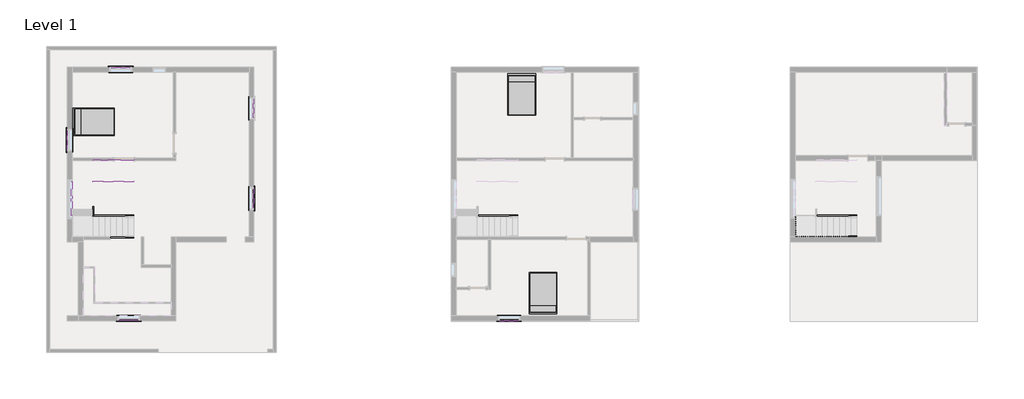
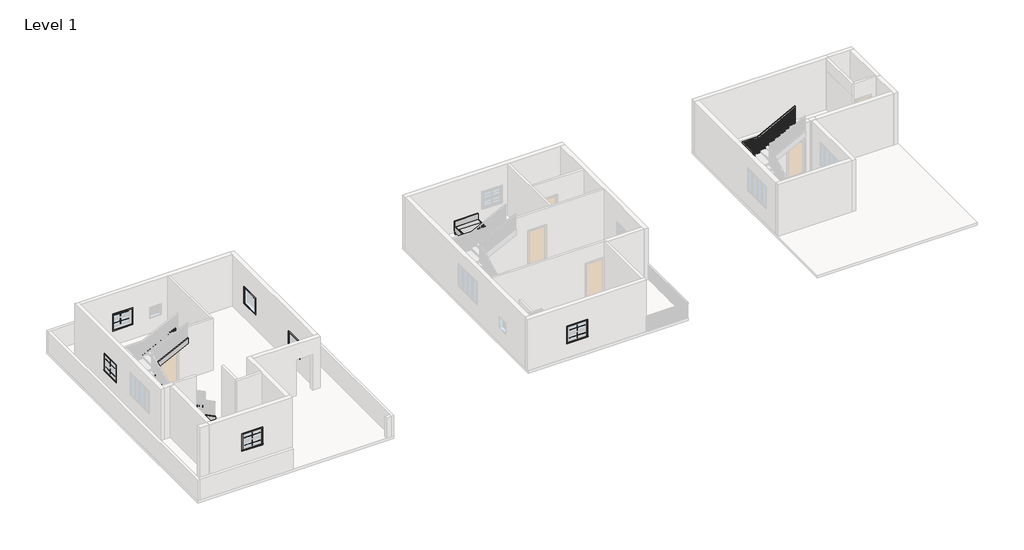
# One storey, part 7 of 8: 22 proxies, 10 members, 3 furniture elements, 1 railing.
"""IFC4 building model written with IfcOpenShell, lengths in millimetres."""

from ifc_helpers import new_model, si_unit, frame, origin, place, context, project, spatial, polyline, outline, extrude, faceted_brep, transform, mapped, element, save
from components import muntin_pattern_2x2_muntin_pattern_2x2_4e6d5dbc, muntin_pattern_2x2_muntin_pattern_2x2_9ec9cf3e, trim_window_exterior_flat_with_sill_79aa6636, trim_window_interior_flat_picture_frame_55a9d760, bed_17739_bed_17739_15c61121

model = new_model("IFC4")

# Units and contexts
model_context = context("Model", 3, world=origin())
ifc_project = project(units=[si_unit("LENGTHUNIT", "METRE", prefix="MILLI")], contexts=[model_context])

# Site, building, storey
site = spatial("IfcSite", under=ifc_project)
building = spatial("IfcBuilding", under=site)
storey = spatial("IfcBuildingStorey", under=building, Name="Level 1", Elevation=0.0)

# Proxies
placement = place(None, origin())
muntin_pattern_2x2_muntin_pattern_2x2_shape = muntin_pattern_2x2_muntin_pattern_2x2_4e6d5dbc(model_context)
element("IfcBuildingElementProxy", 1, Name="Muntin Pattern_2x2 : Muntin Pattern_2x2", ObjectType="Muntin Pattern_2x2 : Muntin Pattern_2x2", at=placement, inside=storey, context=model_context, shape_type="MappedRepresentation", body=[
    mapped(muntin_pattern_2x2_muntin_pattern_2x2_shape, transform((-22935.3539184, 3510.7100713, 1441.45), x_axis=(0.0, 1.0, 0.0), y_axis=(-1.0, 0.0, 0.0), z_axis=(0.0, 0.0, 1.0))),
])
element("IfcBuildingElementProxy", 2, Name="Muntin Pattern_2x2 : Muntin Pattern_2x2", ObjectType="Muntin Pattern_2x2 : Muntin Pattern_2x2", at=placement, inside=storey, context=model_context, shape_type="MappedRepresentation", body=[
    mapped(muntin_pattern_2x2_muntin_pattern_2x2_shape, transform((-20392.1789184, 6987.3350713, 1441.45), x_axis=(1.0, 0.0, 0.0), y_axis=(0.0, 1.0, 0.0), z_axis=(0.0, 0.0, 1.0))),
])
element("IfcBuildingElementProxy", 3, Name="Muntin Pattern_2x2 : Muntin Pattern_2x2", ObjectType="Muntin Pattern_2x2 : Muntin Pattern_2x2", at=placement, inside=storey, context=model_context, shape_type="MappedRepresentation", body=[
    mapped(muntin_pattern_2x2_muntin_pattern_2x2_shape, transform((-14039.0039184, 5028.3600713, 1441.45), x_axis=(0.0, -1.0, 0.0), y_axis=(1.0, 0.0, 0.0), z_axis=(0.0, 0.0, 1.0))),
])
element("IfcBuildingElementProxy", 4, Name="Muntin Pattern_2x2 : Muntin Pattern_2x2", ObjectType="Muntin Pattern_2x2 : Muntin Pattern_2x2", at=placement, inside=storey, context=model_context, shape_type="MappedRepresentation", body=[
    mapped(muntin_pattern_2x2_muntin_pattern_2x2_shape, transform((-14039.0039184, 723.0600713, 1441.45), x_axis=(0.0, -1.0, 0.0), y_axis=(1.0, 0.0, 0.0), z_axis=(0.0, 0.0, 1.0))),
])
element("IfcBuildingElementProxy", 5, Name="Muntin Pattern_2x2 : Muntin Pattern_2x2", ObjectType="Muntin Pattern_2x2 : Muntin Pattern_2x2", at=placement, inside=storey, context=model_context, shape_type="MappedRepresentation", body=[
    mapped(muntin_pattern_2x2_muntin_pattern_2x2_shape, transform((-20011.1789184, -5109.4149287, 1441.45), x_axis=(-1.0, 0.0, 0.0), y_axis=(0.0, -1.0, 0.0), z_axis=(0.0, 0.0, 1.0))),
])
element("IfcBuildingElementProxy", 6, Name="Muntin Pattern_2x2 : Muntin Pattern_2x2", ObjectType="Muntin Pattern_2x2 : Muntin Pattern_2x2", at=placement, inside=storey, context=model_context, shape_type="MappedRepresentation", body=[
    mapped(muntin_pattern_2x2_muntin_pattern_2x2_shape, transform((-1847.2308482, -5109.4149287, 1441.45), x_axis=(-1.0, 0.0, 0.0), y_axis=(0.0, -1.0, 0.0), z_axis=(0.0, 0.0, 1.0))),
])
muntin_pattern_2x2_muntin_pattern_2x2_2_shape = muntin_pattern_2x2_muntin_pattern_2x2_9ec9cf3e(model_context)
element("IfcBuildingElementProxy", 7, Name="Muntin Pattern_2x2 : Muntin Pattern_2x2", ObjectType="Muntin Pattern_2x2 : Muntin Pattern_2x2", at=placement, inside=storey, context=model_context, shape_type="MappedRepresentation", body=[
    mapped(muntin_pattern_2x2_muntin_pattern_2x2_2_shape, transform((-22935.3539184, 3510.7100713, 984.25), x_axis=(0.0, 1.0, 0.0), y_axis=(-1.0, 0.0, 0.0), z_axis=(0.0, 0.0, 1.0))),
])
element("IfcBuildingElementProxy", 8, Name="Muntin Pattern_2x2 : Muntin Pattern_2x2", ObjectType="Muntin Pattern_2x2 : Muntin Pattern_2x2", at=placement, inside=storey, context=model_context, shape_type="MappedRepresentation", body=[
    mapped(muntin_pattern_2x2_muntin_pattern_2x2_2_shape, transform((-20392.1789184, 6987.3350713, 984.25), x_axis=(1.0, 0.0, 0.0), y_axis=(0.0, 1.0, 0.0), z_axis=(0.0, 0.0, 1.0))),
])
element("IfcBuildingElementProxy", 9, Name="Muntin Pattern_2x2 : Muntin Pattern_2x2", ObjectType="Muntin Pattern_2x2 : Muntin Pattern_2x2", at=placement, inside=storey, context=model_context, shape_type="MappedRepresentation", body=[
    mapped(muntin_pattern_2x2_muntin_pattern_2x2_2_shape, transform((-14039.0039184, 723.0600713, 984.25), x_axis=(0.0, -1.0, 0.0), y_axis=(1.0, 0.0, 0.0), z_axis=(0.0, 0.0, 1.0))),
])
element("IfcBuildingElementProxy", 10, Name="Muntin Pattern_2x2 : Muntin Pattern_2x2", ObjectType="Muntin Pattern_2x2 : Muntin Pattern_2x2", at=placement, inside=storey, context=model_context, shape_type="MappedRepresentation", body=[
    mapped(muntin_pattern_2x2_muntin_pattern_2x2_2_shape, transform((-20011.1789184, -5109.4149287, 984.25), x_axis=(-1.0, 0.0, 0.0), y_axis=(0.0, -1.0, 0.0), z_axis=(0.0, 0.0, 1.0))),
])
element("IfcBuildingElementProxy", 11, Name="Muntin Pattern_2x2 : Muntin Pattern_2x2", ObjectType="Muntin Pattern_2x2 : Muntin Pattern_2x2", at=placement, inside=storey, context=model_context, shape_type="MappedRepresentation", body=[
    mapped(muntin_pattern_2x2_muntin_pattern_2x2_2_shape, transform((-1847.2308482, -5109.4149287, 984.25), x_axis=(-1.0, 0.0, 0.0), y_axis=(0.0, -1.0, 0.0), z_axis=(0.0, 0.0, 1.0))),
])
trim_window_exterior_flat_with_sill_shape = trim_window_exterior_flat_with_sill_79aa6636(model_context)
element("IfcBuildingElementProxy", 12, Name="Trim-Window-Exterior-Flat : with Sill", ObjectType="Trim-Window-Exterior-Flat : with Sill", at=placement, inside=storey, context=model_context, shape_type="MappedRepresentation", body=[
    mapped(trim_window_exterior_flat_with_sill_shape, transform((-22944.8789184, 3510.7100713, 1828.8), x_axis=(0.0, -1.0, 0.0), y_axis=(0.0, 0.0, 1.0), z_axis=(-1.0, 0.0, 0.0))),
])
element("IfcBuildingElementProxy", 13, Name="Trim-Window-Exterior-Flat : with Sill", ObjectType="Trim-Window-Exterior-Flat : with Sill", at=placement, inside=storey, context=model_context, shape_type="MappedRepresentation", body=[
    mapped(trim_window_exterior_flat_with_sill_shape, transform((-20392.1789184, 6996.8600713, 1828.8), x_axis=(-1.0, 0.0, 0.0), y_axis=(0.0, 0.0, 1.0), z_axis=(0.0, 1.0, 0.0))),
])
element("IfcBuildingElementProxy", 14, Name="Trim-Window-Exterior-Flat : with Sill", ObjectType="Trim-Window-Exterior-Flat : with Sill", at=placement, inside=storey, context=model_context, shape_type="MappedRepresentation", body=[
    mapped(trim_window_exterior_flat_with_sill_shape, transform((-14029.4789184, 723.0600713, 1828.8), x_axis=(0.0, 1.0, 0.0), y_axis=(0.0, 0.0, 1.0), z_axis=(1.0, 0.0, 0.0))),
])
element("IfcBuildingElementProxy", 15, Name="Trim-Window-Exterior-Flat : with Sill", ObjectType="Trim-Window-Exterior-Flat : with Sill", at=placement, inside=storey, context=model_context, shape_type="MappedRepresentation", body=[
    mapped(trim_window_exterior_flat_with_sill_shape, transform((-20011.1789184, -5118.9399287, 1828.8), x_axis=(1.0, 0.0, 0.0), y_axis=(0.0, 0.0, 1.0), z_axis=(0.0, -1.0, 0.0))),
])
element("IfcBuildingElementProxy", 16, Name="Trim-Window-Exterior-Flat : with Sill", ObjectType="Trim-Window-Exterior-Flat : with Sill", at=placement, inside=storey, context=model_context, shape_type="MappedRepresentation", body=[
    mapped(trim_window_exterior_flat_with_sill_shape, transform((-1847.2308482, -5118.9399287, 1828.8), x_axis=(1.0, 0.0, 0.0), y_axis=(0.0, 0.0, 1.0), z_axis=(0.0, -1.0, 0.0))),
])
trim_window_interior_flat_picture_frame_shape = trim_window_interior_flat_picture_frame_55a9d760(model_context)
element("IfcBuildingElementProxy", 17, Name="Trim-Window-Interior-Flat : Picture Frame", ObjectType="Trim-Window-Interior-Flat : Picture Frame", at=placement, inside=storey, context=model_context, shape_type="MappedRepresentation", body=[
    mapped(trim_window_interior_flat_picture_frame_shape, transform((-22716.2789184, 3510.7100713, 1828.8), x_axis=(0.0, 1.0, 0.0), y_axis=(0.0, 0.0, 1.0), z_axis=(1.0, 0.0, 0.0))),
])
element("IfcBuildingElementProxy", 18, Name="Trim-Window-Interior-Flat : Picture Frame", ObjectType="Trim-Window-Interior-Flat : Picture Frame", at=placement, inside=storey, context=model_context, shape_type="MappedRepresentation", body=[
    mapped(trim_window_interior_flat_picture_frame_shape, transform((-20392.1789184, 6768.2600713, 1828.8), x_axis=(1.0, 0.0, 0.0), y_axis=(0.0, 0.0, 1.0), z_axis=(0.0, -1.0, 0.0))),
])
element("IfcBuildingElementProxy", 19, Name="Trim-Window-Interior-Flat : Picture Frame", ObjectType="Trim-Window-Interior-Flat : Picture Frame", at=placement, inside=storey, context=model_context, shape_type="MappedRepresentation", body=[
    mapped(trim_window_interior_flat_picture_frame_shape, transform((-14258.0789184, 5028.3600713, 1828.8), x_axis=(0.0, -1.0, 0.0), y_axis=(0.0, 0.0, 1.0), z_axis=(-1.0, 0.0, 0.0))),
])
element("IfcBuildingElementProxy", 20, Name="Trim-Window-Interior-Flat : Picture Frame", ObjectType="Trim-Window-Interior-Flat : Picture Frame", at=placement, inside=storey, context=model_context, shape_type="MappedRepresentation", body=[
    mapped(trim_window_interior_flat_picture_frame_shape, transform((-14258.0789184, 723.0600713, 1828.8), x_axis=(0.0, -1.0, 0.0), y_axis=(0.0, 0.0, 1.0), z_axis=(-1.0, 0.0, 0.0))),
])
element("IfcBuildingElementProxy", 21, Name="Trim-Window-Interior-Flat : Picture Frame", ObjectType="Trim-Window-Interior-Flat : Picture Frame", at=placement, inside=storey, context=model_context, shape_type="MappedRepresentation", body=[
    mapped(trim_window_interior_flat_picture_frame_shape, transform((-20011.1789184, -4890.3399287, 1828.8), x_axis=(-1.0, 0.0, 0.0), y_axis=(0.0, 0.0, 1.0), z_axis=(0.0, 1.0, 0.0))),
])
element("IfcBuildingElementProxy", 22, Name="Trim-Window-Interior-Flat : Picture Frame", ObjectType="Trim-Window-Interior-Flat : Picture Frame", at=placement, inside=storey, context=model_context, shape_type="MappedRepresentation", body=[
    mapped(trim_window_interior_flat_picture_frame_shape, transform((-1847.2308482, -4890.3399287, 1828.8), x_axis=(-1.0, 0.0, 0.0), y_axis=(0.0, 0.0, 1.0), z_axis=(0.0, 1.0, 0.0))),
])

# Furniture
bed_17739_bed_17739_shape = bed_17739_bed_17739_15c61121(model_context)
element("IfcFurniture", 23, ObjectType="Bed_17739 : Bed_17739", at=placement, inside=storey, context=model_context, shape_type="MappedRepresentation", body=[
    mapped(bed_17739_bed_17739_shape, transform((-21662.1789184, 4380.6600713, 0.0), x_axis=(0.0, 1.0, 0.0), y_axis=(-1.0, 0.0, 0.0), z_axis=(0.0, 0.0, 1.0))),
])
element("IfcFurniture", 24, ObjectType="Bed_17739 : Bed_17739", at=placement, inside=storey, context=model_context, shape_type="MappedRepresentation", body=[
    mapped(bed_17739_bed_17739_shape, transform((-221.6308482, -3785.4399287, 0.0), x_axis=(-1.0, 0.0, 0.0), y_axis=(0.0, -1.0, 0.0), z_axis=(0.0, 0.0, 1.0))),
])
element("IfcFurniture", 25, ObjectType="Bed_17739 : Bed_17739", at=placement, inside=storey, context=model_context, shape_type="MappedRepresentation", body=[
    mapped(bed_17739_bed_17739_shape, transform((-1243.9808482, 5663.3600713, 0.0), x_axis=(1.0, 0.0, 0.0), y_axis=(0.0, 1.0, 0.0), z_axis=(0.0, 0.0, 1.0))),
])

# Members
element("IfcMember", 26, ObjectType="Stringer - 2\" Width", at=placement, inside=storey, context=model_context, shape_type="SweptSolid", body=[
    extrude(outline(polyline([(0.0, -1428.1308482), (202.7933564, -1428.1308482), (819.9503812, -2672.7308482), (819.9503812, -3358.8318192), (0.0, -1705.2652172), (0.0, -1428.1308482)])), frame((0.0, -1169.2399287, 0.0), z_axis=(0.0, 1.0, 0.0), x_axis=(0.0, 0.0, 1.0)), (0.0, 0.0, 1.0), 50.8),
])
element("IfcMember", 27, ObjectType="Stringer - 2\" Width", at=placement, inside=storey, context=model_context, shape_type="SweptSolid", body=[
    extrude(outline(polyline([(0.0, -1428.1308482), (202.7933564, -1428.1308482), (1147.4214556, -3333.1308482), (807.206098, -3333.1308482), (0.0, -1705.2652172), (0.0, -1428.1308482)])), frame((0.0, -127.8399287, 0.0), z_axis=(0.0, 1.0, 0.0), x_axis=(0.0, 0.0, 1.0)), (0.0, 0.0, 1.0), 50.8),
])
element("IfcMember", 28, ObjectType="Stringer - 2\" Width", at=placement, inside=storey, context=model_context, shape_type="SweptSolid", body=[
    extrude(outline(polyline([(0.0, -19769.8789184), (202.7933564, -19769.8789184), (819.9503812, -21014.4789184), (819.9503812, -21700.5798894), (0.0, -20047.0132874), (0.0, -19769.8789184)])), frame((0.0, -1169.2399287, 0.0), z_axis=(0.0, 1.0, 0.0), x_axis=(0.0, 0.0, 1.0)), (0.0, 0.0, 1.0), 50.8),
])
element("IfcMember", 29, ObjectType="Stringer - 2\" Width", at=placement, inside=storey, context=model_context, shape_type="SweptSolid", body=[
    extrude(outline(polyline([(-102.7408997, 1323.6027923), (837.3600713, 1789.768563), (1523.4610422, 1789.768563), (583.3600713, 1323.6027923), (-102.7408997, 1323.6027923)])), frame((-22767.0789184, 0.0, 0.0), z_axis=(1.0, 0.0, 0.0), x_axis=(0.0, 1.0, 0.0)), (0.0, 0.0, 1.0), 50.8),
])
element("IfcMember", 30, ObjectType="Stringer - 2\" Width", at=placement, inside=storey, context=model_context, shape_type="SweptSolid", body=[
    extrude(outline(polyline([(2293.4209741, -21014.4789184), (2910.5779989, -19769.8789184), (3250.7933564, -19769.8789184), (2293.4209741, -21700.5798894), (2293.4209741, -21014.4789184)])), frame((0.0, 2539.1600713, 0.0), z_axis=(0.0, 1.0, 0.0), x_axis=(0.0, 0.0, 1.0)), (0.0, 0.0, 1.0), 50.8),
])
element("IfcMember", 31, ObjectType="Stringer - 2\" Width", at=placement, inside=storey, context=model_context, shape_type="SweptSolid", body=[
    extrude(outline(polyline([(0.0, -19769.8789184), (202.7933564, -19769.8789184), (1147.4214556, -21674.8789184), (807.206098, -21674.8789184), (0.0, -20047.0132874), (0.0, -19769.8789184)])), frame((0.0, -127.8399287, 0.0), z_axis=(0.0, 1.0, 0.0), x_axis=(0.0, 0.0, 1.0)), (0.0, 0.0, 1.0), 50.8),
])
element("IfcMember", 32, ObjectType="Stringer - 2\" Width", at=placement, inside=storey, context=model_context, shape_type="SweptSolid", body=[
    extrude(outline(polyline([(-127.8399287, 970.9416352), (-127.8399287, 1311.1569927), (1497.7600713, 2117.2396374), (1497.7600713, 1777.0242799), (-127.8399287, 970.9416352)])), frame((-21725.6789184, 0.0, 0.0), z_axis=(1.0, 0.0, 0.0), x_axis=(0.0, 1.0, 0.0)), (0.0, 0.0, 1.0), 50.8),
])
element("IfcMember", 33, ObjectType="Stringer - 2\" Width", at=placement, inside=storey, context=model_context, shape_type="SweptSolid", body=[
    extrude(outline(polyline([(2280.9751746, -21725.6789184), (1940.759817, -21725.6789184), (2910.5779989, -19769.8789184), (3250.7933564, -19769.8789184), (2280.9751746, -21725.6789184)])), frame((0.0, 1497.7600713, 0.0), z_axis=(0.0, 1.0, 0.0), x_axis=(0.0, 0.0, 1.0)), (0.0, 0.0, 1.0), 50.8),
])
element("IfcMember", 34, ObjectType="Stringer - 2\" Width", at=placement, inside=storey, context=model_context, shape_type="SweptSolid", body=[
    extrude(outline(polyline([(0.0, 14750.242447), (204.6227955, 14750.242447), (851.1682501, 13505.642447), (851.1682501, 12844.4564917), (0.0, 14482.955373), (0.0, 14750.242447)])), frame((0.0, -1169.2399287, 0.0), z_axis=(0.0, 1.0, 0.0), x_axis=(0.0, 0.0, 1.0)), (0.0, 0.0, 1.0), 50.8),
])
element("IfcMember", 35, ObjectType="Stringer - 2\" Width", at=placement, inside=storey, context=model_context, shape_type="SweptSolid", body=[
    extrude(outline(polyline([(0.0, 14750.242447), (204.6227955, 14750.242447), (1194.2331851, 12845.242447), (850.7599615, 12845.242447), (0.0, 14482.955373), (0.0, 14750.242447)])), frame((0.0, -127.8399287, 0.0), z_axis=(0.0, 1.0, 0.0), x_axis=(0.0, 0.0, 1.0)), (0.0, 0.0, 1.0), 50.8),
])

# Railing
element("IfcRailing", 36, ObjectType="Handrail - Rectangular", at=placement, inside=storey, context=model_context, shape_type="SolidModel", body=[
    faceted_brep([(14750.242447, -1118.4399287, 1059.5428571), (14750.242447, -1118.4399287, 1002.2973199), (14750.242447, -1067.6399287, 1002.2973199), (14750.242447, -1067.6399287, 1059.5428571), (12654.742447, -1118.4399287, 2148.1142857), (12642.3347878, -1118.4399287, 2097.3142857), (12642.3347878, -1067.6399287, 2097.3142857), (12654.742447, -1067.6399287, 2148.1142857), (11803.842447, -1118.4399287, 2097.3142857), (11803.842447, -1118.4399287, 2148.1142857), (11803.842447, -267.5399287, 2148.1142857), (11803.842447, -255.1322695, 2097.3142857), (11854.642447, -1067.6399287, 2097.3142857), (11854.642447, -255.1322695, 2097.3142857), (11854.642447, -1067.6399287, 2148.1142857), (11854.642447, -267.5399287, 2148.1142857), (11803.842447, 2539.1600713, 3113.3142857), (11803.842447, 2539.1600713, 3164.1142857), (12654.742447, 2539.1600713, 3164.1142857), (12667.1501063, 2539.1600713, 3113.3142857), (11854.642447, 2488.3600713, 3113.3142857), (12667.1501063, 2488.3600713, 3113.3142857), (11854.642447, 2488.3600713, 3164.1142857), (12654.742447, 2488.3600713, 3164.1142857), (11803.842447, 1688.2600713, 3164.1142857), (11803.842447, 1700.6677305, 3113.3142857), (11854.642447, 1700.6677305, 3113.3142857), (11854.642447, 1688.2600713, 3164.1142857), (14750.242447, 2539.1600713, 4252.6857143), (14750.242447, 2488.3600713, 4252.6857143), (14750.242447, 2488.3600713, 4195.440177), (14750.242447, 2539.1600713, 4195.440177)], [[[0, 1, 2, 3]], [[1, 0, 4, 5]], [[2, 1, 5, 6]], [[3, 2, 6, 7]], [[0, 3, 7, 4]], [[8, 9, 10, 11]], [[12, 8, 11, 13]], [[14, 12, 13, 15]], [[9, 14, 15, 10]], [[16, 17, 18, 19]], [[20, 16, 19, 21]], [[22, 20, 21, 23]], [[17, 22, 23, 18]], [[5, 4, 9, 8]], [[6, 5, 8, 12]], [[7, 6, 12, 14]], [[4, 7, 14, 9]], [[11, 10, 24, 25]], [[13, 11, 25, 26]], [[15, 13, 26, 27]], [[10, 15, 27, 24]], [[25, 24, 17, 16]], [[26, 25, 16, 20]], [[27, 26, 20, 22]], [[24, 27, 22, 17]], [[28, 29, 30, 31]], [[19, 18, 28, 31]], [[21, 19, 31, 30]], [[23, 21, 30, 29]], [[18, 23, 29, 28]]]),
    extrude(outline(polyline([(4150.9077095, 14664.517447), (3193.1428571, 14664.517447), (3193.1428571, 14683.567447), (4160.8038134, 14683.567447), (4150.9077095, 14664.517447)])), frame((0.0, 2504.2350713, 0.0), z_axis=(0.0, 1.0, 0.0), x_axis=(0.0, 0.0, 1.0)), (0.0, 0.0, 1.0), 19.05),
    extrude(outline(polyline([(4098.1284887, 14562.917447), (3193.1428571, 14562.917447), (3193.1428571, 14581.967447), (4108.0245926, 14581.967447), (4098.1284887, 14562.917447)])), frame((0.0, 2504.2350713, 0.0), z_axis=(0.0, 1.0, 0.0), x_axis=(0.0, 0.0, 1.0)), (0.0, 0.0, 1.0), 19.05),
    extrude(outline(polyline([(4045.3492679, 14461.317447), (3193.1428571, 14461.317447), (3193.1428571, 14480.367447), (4055.2453718, 14480.367447), (4045.3492679, 14461.317447)])), frame((0.0, 2504.2350713, 0.0), z_axis=(0.0, 1.0, 0.0), x_axis=(0.0, 0.0, 1.0)), (0.0, 0.0, 1.0), 19.05),
    extrude(outline(polyline([(3992.5700472, 14359.717447), (3048.0, 14359.717447), (3048.0, 14378.767447), (4002.466151, 14378.767447), (3992.5700472, 14359.717447)])), frame((0.0, 2504.2350713, 0.0), z_axis=(0.0, 1.0, 0.0), x_axis=(0.0, 0.0, 1.0)), (0.0, 0.0, 1.0), 19.05),
    extrude(outline(polyline([(3939.7908264, 14258.117447), (3048.0, 14258.117447), (3048.0, 14277.167447), (3949.6869303, 14277.167447), (3939.7908264, 14258.117447)])), frame((0.0, 2504.2350713, 0.0), z_axis=(0.0, 1.0, 0.0), x_axis=(0.0, 0.0, 1.0)), (0.0, 0.0, 1.0), 19.05),
    extrude(outline(polyline([(3887.0116056, 14156.517447), (2902.8571429, 14156.517447), (2902.8571429, 14175.567447), (3896.9077095, 14175.567447), (3887.0116056, 14156.517447)])), frame((0.0, 2504.2350713, 0.0), z_axis=(0.0, 1.0, 0.0), x_axis=(0.0, 0.0, 1.0)), (0.0, 0.0, 1.0), 19.05),
    extrude(outline(polyline([(3834.2323848, 14054.917447), (2902.8571429, 14054.917447), (2902.8571429, 14073.967447), (3844.1284887, 14073.967447), (3834.2323848, 14054.917447)])), frame((0.0, 2504.2350713, 0.0), z_axis=(0.0, 1.0, 0.0), x_axis=(0.0, 0.0, 1.0)), (0.0, 0.0, 1.0), 19.05),
    extrude(outline(polyline([(3781.453164, 13953.317447), (2902.8571429, 13953.317447), (2902.8571429, 13972.367447), (3791.3492679, 13972.367447), (3781.453164, 13953.317447)])), frame((0.0, 2504.2350713, 0.0), z_axis=(0.0, 1.0, 0.0), x_axis=(0.0, 0.0, 1.0)), (0.0, 0.0, 1.0), 19.05),
    extrude(outline(polyline([(3728.6739433, 13851.717447), (2757.7142857, 13851.717447), (2757.7142857, 13870.767447), (3738.5700472, 13870.767447), (3728.6739433, 13851.717447)])), frame((0.0, 2504.2350713, 0.0), z_axis=(0.0, 1.0, 0.0), x_axis=(0.0, 0.0, 1.0)), (0.0, 0.0, 1.0), 19.05),
    extrude(outline(polyline([(3675.8947225, 13750.117447), (2757.7142857, 13750.117447), (2757.7142857, 13769.167447), (3685.7908264, 13769.167447), (3675.8947225, 13750.117447)])), frame((0.0, 2504.2350713, 0.0), z_axis=(0.0, 1.0, 0.0), x_axis=(0.0, 0.0, 1.0)), (0.0, 0.0, 1.0), 19.05),
    extrude(outline(polyline([(3623.1155017, 13648.517447), (2757.7142857, 13648.517447), (2757.7142857, 13667.567447), (3633.0116056, 13667.567447), (3623.1155017, 13648.517447)])), frame((0.0, 2504.2350713, 0.0), z_axis=(0.0, 1.0, 0.0), x_axis=(0.0, 0.0, 1.0)), (0.0, 0.0, 1.0), 19.05),
    extrude(outline(polyline([(3570.3362809, 13546.917447), (2612.5714286, 13546.917447), (2612.5714286, 13565.967447), (3580.2323848, 13565.967447), (3570.3362809, 13546.917447)])), frame((0.0, 2504.2350713, 0.0), z_axis=(0.0, 1.0, 0.0), x_axis=(0.0, 0.0, 1.0)), (0.0, 0.0, 1.0), 19.05),
    extrude(outline(polyline([(3517.5570601, 13445.317447), (2612.5714286, 13445.317447), (2612.5714286, 13464.367447), (3527.453164, 13464.367447), (3517.5570601, 13445.317447)])), frame((0.0, 2504.2350713, 0.0), z_axis=(0.0, 1.0, 0.0), x_axis=(0.0, 0.0, 1.0)), (0.0, 0.0, 1.0), 19.05),
    extrude(outline(polyline([(3464.7778394, 13343.717447), (2612.5714286, 13343.717447), (2612.5714286, 13362.767447), (3474.6739433, 13362.767447), (3464.7778394, 13343.717447)])), frame((0.0, 2504.2350713, 0.0), z_axis=(0.0, 1.0, 0.0), x_axis=(0.0, 0.0, 1.0)), (0.0, 0.0, 1.0), 19.05),
    extrude(outline(polyline([(3411.9986186, 13242.117447), (2467.4285714, 13242.117447), (2467.4285714, 13261.167447), (3421.8947225, 13261.167447), (3411.9986186, 13242.117447)])), frame((0.0, 2504.2350713, 0.0), z_axis=(0.0, 1.0, 0.0), x_axis=(0.0, 0.0, 1.0)), (0.0, 0.0, 1.0), 19.05),
    extrude(outline(polyline([(3359.2193978, 13140.517447), (2467.4285714, 13140.517447), (2467.4285714, 13159.567447), (3369.1155017, 13159.567447), (3359.2193978, 13140.517447)])), frame((0.0, 2504.2350713, 0.0), z_axis=(0.0, 1.0, 0.0), x_axis=(0.0, 0.0, 1.0)), (0.0, 0.0, 1.0), 19.05),
    extrude(outline(polyline([(3306.440177, 13038.917447), (2322.2857143, 13038.917447), (2322.2857143, 13057.967447), (3316.3362809, 13057.967447), (3306.440177, 13038.917447)])), frame((0.0, 2504.2350713, 0.0), z_axis=(0.0, 1.0, 0.0), x_axis=(0.0, 0.0, 1.0)), (0.0, 0.0, 1.0), 19.05),
    extrude(outline(polyline([(3253.6609562, 12937.317447), (2322.2857143, 12937.317447), (2322.2857143, 12956.367447), (3263.5570601, 12956.367447), (3253.6609562, 12937.317447)])), frame((0.0, 2504.2350713, 0.0), z_axis=(0.0, 1.0, 0.0), x_axis=(0.0, 0.0, 1.0)), (0.0, 0.0, 1.0), 19.05),
    extrude(outline(polyline([(3200.8817355, 12835.717447), (2322.2857143, 12835.717447), (2322.2857143, 12854.767447), (3210.7778394, 12854.767447), (3200.8817355, 12835.717447)])), frame((0.0, 2504.2350713, 0.0), z_axis=(0.0, 1.0, 0.0), x_axis=(0.0, 0.0, 1.0)), (0.0, 0.0, 1.0), 19.05),
    extrude(outline(polyline([(3148.1025147, 12734.117447), (2177.1428571, 12734.117447), (2177.1428571, 12753.167447), (3157.9986186, 12753.167447), (3148.1025147, 12734.117447)])), frame((0.0, 2504.2350713, 0.0), z_axis=(0.0, 1.0, 0.0), x_axis=(0.0, 0.0, 1.0)), (0.0, 0.0, 1.0), 19.05),
    extrude(outline(polyline([(12632.517447, 2523.2850713), (12651.567447, 2523.2850713), (12651.567447, 2504.2350713), (12632.517447, 2504.2350713), (12632.517447, 2523.2850713)])), frame((0.0, 0.0, 2177.1428571), z_axis=(0.0, 0.0, 1.0), x_axis=(1.0, 0.0, 0.0)), (0.0, 0.0, 1.0), 936.1714286),
    extrude(outline(polyline([(12530.917447, 2523.2850713), (12549.967447, 2523.2850713), (12549.967447, 2504.2350713), (12530.917447, 2504.2350713), (12530.917447, 2523.2850713)])), frame((0.0, 0.0, 2177.1428571), z_axis=(0.0, 0.0, 1.0), x_axis=(1.0, 0.0, 0.0)), (0.0, 0.0, 1.0), 936.1714286),
    extrude(outline(polyline([(12429.317447, 2523.2850713), (12448.367447, 2523.2850713), (12448.367447, 2504.2350713), (12429.317447, 2504.2350713), (12429.317447, 2523.2850713)])), frame((0.0, 0.0, 2177.1428571), z_axis=(0.0, 0.0, 1.0), x_axis=(1.0, 0.0, 0.0)), (0.0, 0.0, 1.0), 936.1714286),
    extrude(outline(polyline([(12327.717447, 2523.2850713), (12346.767447, 2523.2850713), (12346.767447, 2504.2350713), (12327.717447, 2504.2350713), (12327.717447, 2523.2850713)])), frame((0.0, 0.0, 2177.1428571), z_axis=(0.0, 0.0, 1.0), x_axis=(1.0, 0.0, 0.0)), (0.0, 0.0, 1.0), 936.1714286),
    extrude(outline(polyline([(12226.117447, 2523.2850713), (12245.167447, 2523.2850713), (12245.167447, 2504.2350713), (12226.117447, 2504.2350713), (12226.117447, 2523.2850713)])), frame((0.0, 0.0, 2177.1428571), z_axis=(0.0, 0.0, 1.0), x_axis=(1.0, 0.0, 0.0)), (0.0, 0.0, 1.0), 936.1714286),
    extrude(outline(polyline([(12124.517447, 2523.2850713), (12143.567447, 2523.2850713), (12143.567447, 2504.2350713), (12124.517447, 2504.2350713), (12124.517447, 2523.2850713)])), frame((0.0, 0.0, 2177.1428571), z_axis=(0.0, 0.0, 1.0), x_axis=(1.0, 0.0, 0.0)), (0.0, 0.0, 1.0), 936.1714286),
    extrude(outline(polyline([(12022.917447, 2523.2850713), (12041.967447, 2523.2850713), (12041.967447, 2504.2350713), (12022.917447, 2504.2350713), (12022.917447, 2523.2850713)])), frame((0.0, 0.0, 2177.1428571), z_axis=(0.0, 0.0, 1.0), x_axis=(1.0, 0.0, 0.0)), (0.0, 0.0, 1.0), 936.1714286),
    extrude(outline(polyline([(11921.317447, 2523.2850713), (11940.367447, 2523.2850713), (11940.367447, 2504.2350713), (11921.317447, 2504.2350713), (11921.317447, 2523.2850713)])), frame((0.0, 0.0, 2177.1428571), z_axis=(0.0, 0.0, 1.0), x_axis=(1.0, 0.0, 0.0)), (0.0, 0.0, 1.0), 936.1714286),
    extrude(outline(polyline([(11819.717447, 2453.4350713), (11819.717447, 2472.4850713), (11838.767447, 2472.4850713), (11838.767447, 2453.4350713), (11819.717447, 2453.4350713)])), frame((0.0, 0.0, 2177.1428571), z_axis=(0.0, 0.0, 1.0), x_axis=(1.0, 0.0, 0.0)), (0.0, 0.0, 1.0), 936.1714286),
    extrude(outline(polyline([(11819.717447, 2351.8350713), (11819.717447, 2370.8850713), (11838.767447, 2370.8850713), (11838.767447, 2351.8350713), (11819.717447, 2351.8350713)])), frame((0.0, 0.0, 2177.1428571), z_axis=(0.0, 0.0, 1.0), x_axis=(1.0, 0.0, 0.0)), (0.0, 0.0, 1.0), 936.1714286),
    extrude(outline(polyline([(11819.717447, 2250.2350713), (11819.717447, 2269.2850713), (11838.767447, 2269.2850713), (11838.767447, 2250.2350713), (11819.717447, 2250.2350713)])), frame((0.0, 0.0, 2177.1428571), z_axis=(0.0, 0.0, 1.0), x_axis=(1.0, 0.0, 0.0)), (0.0, 0.0, 1.0), 936.1714286),
    extrude(outline(polyline([(11819.717447, 2148.6350713), (11819.717447, 2167.6850713), (11838.767447, 2167.6850713), (11838.767447, 2148.6350713), (11819.717447, 2148.6350713)])), frame((0.0, 0.0, 2177.1428571), z_axis=(0.0, 0.0, 1.0), x_axis=(1.0, 0.0, 0.0)), (0.0, 0.0, 1.0), 936.1714286),
    extrude(outline(polyline([(11819.717447, 2047.0350713), (11819.717447, 2066.0850713), (11838.767447, 2066.0850713), (11838.767447, 2047.0350713), (11819.717447, 2047.0350713)])), frame((0.0, 0.0, 2177.1428571), z_axis=(0.0, 0.0, 1.0), x_axis=(1.0, 0.0, 0.0)), (0.0, 0.0, 1.0), 936.1714286),
    extrude(outline(polyline([(11819.717447, 1945.4350713), (11819.717447, 1964.4850713), (11838.767447, 1964.4850713), (11838.767447, 1945.4350713), (11819.717447, 1945.4350713)])), frame((0.0, 0.0, 2177.1428571), z_axis=(0.0, 0.0, 1.0), x_axis=(1.0, 0.0, 0.0)), (0.0, 0.0, 1.0), 936.1714286),
    extrude(outline(polyline([(11819.717447, 1843.8350713), (11819.717447, 1862.8850713), (11838.767447, 1862.8850713), (11838.767447, 1843.8350713), (11819.717447, 1843.8350713)])), frame((0.0, 0.0, 2177.1428571), z_axis=(0.0, 0.0, 1.0), x_axis=(1.0, 0.0, 0.0)), (0.0, 0.0, 1.0), 936.1714286),
    extrude(outline(polyline([(11819.717447, 1742.2350713), (11819.717447, 1761.2850713), (11838.767447, 1761.2850713), (11838.767447, 1742.2350713), (11819.717447, 1742.2350713)])), frame((0.0, 0.0, 2177.1428571), z_axis=(0.0, 0.0, 1.0), x_axis=(1.0, 0.0, 0.0)), (0.0, 0.0, 1.0), 936.1714286),
    extrude(outline(polyline([(1659.6850713, 3092.0245926), (1659.6850713, 2177.1428571), (1640.6350713, 2177.1428571), (1640.6350713, 3082.1284887), (1659.6850713, 3092.0245926)])), frame((11819.717447, 0.0, 0.0), z_axis=(1.0, 0.0, 0.0), x_axis=(0.0, 1.0, 0.0)), (0.0, 0.0, 1.0), 19.05),
    extrude(outline(polyline([(1558.0850713, 3039.2453718), (1558.0850713, 2177.1428571), (1539.0350713, 2177.1428571), (1539.0350713, 3029.3492679), (1558.0850713, 3039.2453718)])), frame((11819.717447, 0.0, 0.0), z_axis=(1.0, 0.0, 0.0), x_axis=(0.0, 1.0, 0.0)), (0.0, 0.0, 1.0), 19.05),
    extrude(outline(polyline([(1456.4850713, 2986.466151), (1456.4850713, 2032.0), (1437.4350713, 2032.0), (1437.4350713, 2976.5700472), (1456.4850713, 2986.466151)])), frame((11819.717447, 0.0, 0.0), z_axis=(1.0, 0.0, 0.0), x_axis=(0.0, 1.0, 0.0)), (0.0, 0.0, 1.0), 19.05),
    extrude(outline(polyline([(1354.8850713, 2933.6869303), (1354.8850713, 2032.0), (1335.8350713, 2032.0), (1335.8350713, 2923.7908264), (1354.8850713, 2933.6869303)])), frame((11819.717447, 0.0, 0.0), z_axis=(1.0, 0.0, 0.0), x_axis=(0.0, 1.0, 0.0)), (0.0, 0.0, 1.0), 19.05),
    extrude(outline(polyline([(1253.2850713, 2880.9077095), (1253.2850713, 1886.8571429), (1234.2350713, 1886.8571429), (1234.2350713, 2871.0116056), (1253.2850713, 2880.9077095)])), frame((11819.717447, 0.0, 0.0), z_axis=(1.0, 0.0, 0.0), x_axis=(0.0, 1.0, 0.0)), (0.0, 0.0, 1.0), 19.05),
    extrude(outline(polyline([(1151.6850713, 2828.1284887), (1151.6850713, 1886.8571429), (1132.6350713, 1886.8571429), (1132.6350713, 2818.2323848), (1151.6850713, 2828.1284887)])), frame((11819.717447, 0.0, 0.0), z_axis=(1.0, 0.0, 0.0), x_axis=(0.0, 1.0, 0.0)), (0.0, 0.0, 1.0), 19.05),
    extrude(outline(polyline([(1050.0850713, 2775.3492679), (1050.0850713, 1886.8571429), (1031.0350713, 1886.8571429), (1031.0350713, 2765.453164), (1050.0850713, 2775.3492679)])), frame((11819.717447, 0.0, 0.0), z_axis=(1.0, 0.0, 0.0), x_axis=(0.0, 1.0, 0.0)), (0.0, 0.0, 1.0), 19.05),
    extrude(outline(polyline([(948.4850713, 2722.5700472), (948.4850713, 1741.7142857), (929.4350713, 1741.7142857), (929.4350713, 2712.6739433), (948.4850713, 2722.5700472)])), frame((11819.717447, 0.0, 0.0), z_axis=(1.0, 0.0, 0.0), x_axis=(0.0, 1.0, 0.0)), (0.0, 0.0, 1.0), 19.05),
    extrude(outline(polyline([(846.8850713, 2669.7908264), (846.8850713, 1741.7142857), (827.8350713, 1741.7142857), (827.8350713, 2659.8947225), (846.8850713, 2669.7908264)])), frame((11819.717447, 0.0, 0.0), z_axis=(1.0, 0.0, 0.0), x_axis=(0.0, 1.0, 0.0)), (0.0, 0.0, 1.0), 19.05),
    extrude(outline(polyline([(745.2850713, 2617.0116056), (745.2850713, 1741.7142857), (726.2350713, 1741.7142857), (726.2350713, 2607.1155017), (745.2850713, 2617.0116056)])), frame((11819.717447, 0.0, 0.0), z_axis=(1.0, 0.0, 0.0), x_axis=(0.0, 1.0, 0.0)), (0.0, 0.0, 1.0), 19.05),
    extrude(outline(polyline([(643.6850713, 2564.2323848), (643.6850713, 1596.5714286), (624.6350713, 1596.5714286), (624.6350713, 2554.3362809), (643.6850713, 2564.2323848)])), frame((11819.717447, 0.0, 0.0), z_axis=(1.0, 0.0, 0.0), x_axis=(0.0, 1.0, 0.0)), (0.0, 0.0, 1.0), 19.05),
    extrude(outline(polyline([(542.0850713, 2511.453164), (542.0850713, 1596.5714286), (523.0350713, 1596.5714286), (523.0350713, 2501.5570601), (542.0850713, 2511.453164)])), frame((11819.717447, 0.0, 0.0), z_axis=(1.0, 0.0, 0.0), x_axis=(0.0, 1.0, 0.0)), (0.0, 0.0, 1.0), 19.05),
    extrude(outline(polyline([(440.4850713, 2458.6739433), (440.4850713, 1596.5714286), (421.4350713, 1596.5714286), (421.4350713, 2448.7778394), (440.4850713, 2458.6739433)])), frame((11819.717447, 0.0, 0.0), z_axis=(1.0, 0.0, 0.0), x_axis=(0.0, 1.0, 0.0)), (0.0, 0.0, 1.0), 19.05),
    extrude(outline(polyline([(338.8850713, 2405.8947225), (338.8850713, 1451.4285714), (319.8350713, 1451.4285714), (319.8350713, 2395.9986186), (338.8850713, 2405.8947225)])), frame((11819.717447, 0.0, 0.0), z_axis=(1.0, 0.0, 0.0), x_axis=(0.0, 1.0, 0.0)), (0.0, 0.0, 1.0), 19.05),
    extrude(outline(polyline([(237.2850713, 2353.1155017), (237.2850713, 1451.4285714), (218.2350713, 1451.4285714), (218.2350713, 2343.2193978), (237.2850713, 2353.1155017)])), frame((11819.717447, 0.0, 0.0), z_axis=(1.0, 0.0, 0.0), x_axis=(0.0, 1.0, 0.0)), (0.0, 0.0, 1.0), 19.05),
    extrude(outline(polyline([(135.6850713, 2300.3362809), (135.6850713, 1306.2857143), (116.6350713, 1306.2857143), (116.6350713, 2290.440177), (135.6850713, 2300.3362809)])), frame((11819.717447, 0.0, 0.0), z_axis=(1.0, 0.0, 0.0), x_axis=(0.0, 1.0, 0.0)), (0.0, 0.0, 1.0), 19.05),
    extrude(outline(polyline([(34.0850713, 2247.5570601), (34.0850713, 1306.2857143), (15.0350713, 1306.2857143), (15.0350713, 2237.6609562), (34.0850713, 2247.5570601)])), frame((11819.717447, 0.0, 0.0), z_axis=(1.0, 0.0, 0.0), x_axis=(0.0, 1.0, 0.0)), (0.0, 0.0, 1.0), 19.05),
    extrude(outline(polyline([(-67.5149287, 2194.7778394), (-67.5149287, 1306.2857143), (-86.5649287, 1306.2857143), (-86.5649287, 2184.8817355), (-67.5149287, 2194.7778394)])), frame((11819.717447, 0.0, 0.0), z_axis=(1.0, 0.0, 0.0), x_axis=(0.0, 1.0, 0.0)), (0.0, 0.0, 1.0), 19.05),
    extrude(outline(polyline([(-169.1149287, 2141.9986186), (-169.1149287, 1161.1428571), (-188.1649287, 1161.1428571), (-188.1649287, 2132.1025147), (-169.1149287, 2141.9986186)])), frame((11819.717447, 0.0, 0.0), z_axis=(1.0, 0.0, 0.0), x_axis=(0.0, 1.0, 0.0)), (0.0, 0.0, 1.0), 19.05),
    extrude(outline(polyline([(11819.717447, -289.7649287), (11819.717447, -270.7149287), (11838.767447, -270.7149287), (11838.767447, -289.7649287), (11819.717447, -289.7649287)])), frame((0.0, 0.0, 1161.1428571), z_axis=(0.0, 0.0, 1.0), x_axis=(1.0, 0.0, 0.0)), (0.0, 0.0, 1.0), 936.1714286),
    extrude(outline(polyline([(11819.717447, -391.3649287), (11819.717447, -372.3149287), (11838.767447, -372.3149287), (11838.767447, -391.3649287), (11819.717447, -391.3649287)])), frame((0.0, 0.0, 1161.1428571), z_axis=(0.0, 0.0, 1.0), x_axis=(1.0, 0.0, 0.0)), (0.0, 0.0, 1.0), 936.1714286),
    extrude(outline(polyline([(11819.717447, -492.9649287), (11819.717447, -473.9149287), (11838.767447, -473.9149287), (11838.767447, -492.9649287), (11819.717447, -492.9649287)])), frame((0.0, 0.0, 1161.1428571), z_axis=(0.0, 0.0, 1.0), x_axis=(1.0, 0.0, 0.0)), (0.0, 0.0, 1.0), 936.1714286),
    extrude(outline(polyline([(11819.717447, -594.5649287), (11819.717447, -575.5149287), (11838.767447, -575.5149287), (11838.767447, -594.5649287), (11819.717447, -594.5649287)])), frame((0.0, 0.0, 1161.1428571), z_axis=(0.0, 0.0, 1.0), x_axis=(1.0, 0.0, 0.0)), (0.0, 0.0, 1.0), 936.1714286),
    extrude(outline(polyline([(11819.717447, -696.1649287), (11819.717447, -677.1149287), (11838.767447, -677.1149287), (11838.767447, -696.1649287), (11819.717447, -696.1649287)])), frame((0.0, 0.0, 1161.1428571), z_axis=(0.0, 0.0, 1.0), x_axis=(1.0, 0.0, 0.0)), (0.0, 0.0, 1.0), 936.1714286),
    extrude(outline(polyline([(11819.717447, -797.7649287), (11819.717447, -778.7149287), (11838.767447, -778.7149287), (11838.767447, -797.7649287), (11819.717447, -797.7649287)])), frame((0.0, 0.0, 1161.1428571), z_axis=(0.0, 0.0, 1.0), x_axis=(1.0, 0.0, 0.0)), (0.0, 0.0, 1.0), 936.1714286),
    extrude(outline(polyline([(11819.717447, -899.3649287), (11819.717447, -880.3149287), (11838.767447, -880.3149287), (11838.767447, -899.3649287), (11819.717447, -899.3649287)])), frame((0.0, 0.0, 1161.1428571), z_axis=(0.0, 0.0, 1.0), x_axis=(1.0, 0.0, 0.0)), (0.0, 0.0, 1.0), 936.1714286),
    extrude(outline(polyline([(11819.717447, -1000.9649287), (11819.717447, -981.9149287), (11838.767447, -981.9149287), (11838.767447, -1000.9649287), (11819.717447, -1000.9649287)])), frame((0.0, 0.0, 1161.1428571), z_axis=(0.0, 0.0, 1.0), x_axis=(1.0, 0.0, 0.0)), (0.0, 0.0, 1.0), 936.1714286),
    extrude(outline(polyline([(11914.967447, -1102.5649287), (11895.917447, -1102.5649287), (11895.917447, -1083.5149287), (11914.967447, -1083.5149287), (11914.967447, -1102.5649287)])), frame((0.0, 0.0, 1161.1428571), z_axis=(0.0, 0.0, 1.0), x_axis=(1.0, 0.0, 0.0)), (0.0, 0.0, 1.0), 936.1714286),
    extrude(outline(polyline([(12016.567447, -1102.5649287), (11997.517447, -1102.5649287), (11997.517447, -1083.5149287), (12016.567447, -1083.5149287), (12016.567447, -1102.5649287)])), frame((0.0, 0.0, 1161.1428571), z_axis=(0.0, 0.0, 1.0), x_axis=(1.0, 0.0, 0.0)), (0.0, 0.0, 1.0), 936.1714286),
    extrude(outline(polyline([(12118.167447, -1102.5649287), (12099.117447, -1102.5649287), (12099.117447, -1083.5149287), (12118.167447, -1083.5149287), (12118.167447, -1102.5649287)])), frame((0.0, 0.0, 1161.1428571), z_axis=(0.0, 0.0, 1.0), x_axis=(1.0, 0.0, 0.0)), (0.0, 0.0, 1.0), 936.1714286),
    extrude(outline(polyline([(12219.767447, -1102.5649287), (12200.717447, -1102.5649287), (12200.717447, -1083.5149287), (12219.767447, -1083.5149287), (12219.767447, -1102.5649287)])), frame((0.0, 0.0, 1161.1428571), z_axis=(0.0, 0.0, 1.0), x_axis=(1.0, 0.0, 0.0)), (0.0, 0.0, 1.0), 936.1714286),
    extrude(outline(polyline([(12321.367447, -1102.5649287), (12302.317447, -1102.5649287), (12302.317447, -1083.5149287), (12321.367447, -1083.5149287), (12321.367447, -1102.5649287)])), frame((0.0, 0.0, 1161.1428571), z_axis=(0.0, 0.0, 1.0), x_axis=(1.0, 0.0, 0.0)), (0.0, 0.0, 1.0), 936.1714286),
    extrude(outline(polyline([(12422.967447, -1102.5649287), (12403.917447, -1102.5649287), (12403.917447, -1083.5149287), (12422.967447, -1083.5149287), (12422.967447, -1102.5649287)])), frame((0.0, 0.0, 1161.1428571), z_axis=(0.0, 0.0, 1.0), x_axis=(1.0, 0.0, 0.0)), (0.0, 0.0, 1.0), 936.1714286),
    extrude(outline(polyline([(12524.567447, -1102.5649287), (12505.517447, -1102.5649287), (12505.517447, -1083.5149287), (12524.567447, -1083.5149287), (12524.567447, -1102.5649287)])), frame((0.0, 0.0, 1161.1428571), z_axis=(0.0, 0.0, 1.0), x_axis=(1.0, 0.0, 0.0)), (0.0, 0.0, 1.0), 936.1714286),
    extrude(outline(polyline([(12626.167447, -1102.5649287), (12607.117447, -1102.5649287), (12607.117447, -1083.5149287), (12626.167447, -1083.5149287), (12626.167447, -1102.5649287)])), frame((0.0, 0.0, 1161.1428571), z_axis=(0.0, 0.0, 1.0), x_axis=(1.0, 0.0, 0.0)), (0.0, 0.0, 1.0), 936.1714286),
    extrude(outline(polyline([(2062.8297874, 12708.717447), (1161.1428571, 12708.717447), (1161.1428571, 12727.767447), (2052.9336835, 12727.767447), (2062.8297874, 12708.717447)])), frame((0.0, -1102.5649287, 0.0), z_axis=(0.0, 1.0, 0.0), x_axis=(0.0, 0.0, 1.0)), (0.0, 0.0, 1.0), 19.05),
    extrude(outline(polyline([(2010.0505666, 12810.317447), (1016.0, 12810.317447), (1016.0, 12829.367447), (2000.1544627, 12829.367447), (2010.0505666, 12810.317447)])), frame((0.0, -1102.5649287, 0.0), z_axis=(0.0, 1.0, 0.0), x_axis=(0.0, 0.0, 1.0)), (0.0, 0.0, 1.0), 19.05),
    extrude(outline(polyline([(1957.2713459, 12911.917447), (1016.0, 12911.917447), (1016.0, 12930.967447), (1947.375242, 12930.967447), (1957.2713459, 12911.917447)])), frame((0.0, -1102.5649287, 0.0), z_axis=(0.0, 1.0, 0.0), x_axis=(0.0, 0.0, 1.0)), (0.0, 0.0, 1.0), 19.05),
    extrude(outline(polyline([(1904.4921251, 13013.517447), (1016.0, 13013.517447), (1016.0, 13032.567447), (1894.5960212, 13032.567447), (1904.4921251, 13013.517447)])), frame((0.0, -1102.5649287, 0.0), z_axis=(0.0, 1.0, 0.0), x_axis=(0.0, 0.0, 1.0)), (0.0, 0.0, 1.0), 19.05),
    extrude(outline(polyline([(1851.7129043, 13115.117447), (870.8571429, 13115.117447), (870.8571429, 13134.167447), (1841.8168004, 13134.167447), (1851.7129043, 13115.117447)])), frame((0.0, -1102.5649287, 0.0), z_axis=(0.0, 1.0, 0.0), x_axis=(0.0, 0.0, 1.0)), (0.0, 0.0, 1.0), 19.05),
    extrude(outline(polyline([(1798.9336835, 13216.717447), (870.8571429, 13216.717447), (870.8571429, 13235.767447), (1789.0375796, 13235.767447), (1798.9336835, 13216.717447)])), frame((0.0, -1102.5649287, 0.0), z_axis=(0.0, 1.0, 0.0), x_axis=(0.0, 0.0, 1.0)), (0.0, 0.0, 1.0), 19.05),
    extrude(outline(polyline([(1746.1544627, 13318.317447), (870.8571429, 13318.317447), (870.8571429, 13337.367447), (1736.2583588, 13337.367447), (1746.1544627, 13318.317447)])), frame((0.0, -1102.5649287, 0.0), z_axis=(0.0, 1.0, 0.0), x_axis=(0.0, 0.0, 1.0)), (0.0, 0.0, 1.0), 19.05),
    extrude(outline(polyline([(1693.375242, 13419.917447), (725.7142857, 13419.917447), (725.7142857, 13438.967447), (1683.4791381, 13438.967447), (1693.375242, 13419.917447)])), frame((0.0, -1102.5649287, 0.0), z_axis=(0.0, 1.0, 0.0), x_axis=(0.0, 0.0, 1.0)), (0.0, 0.0, 1.0), 19.05),
    extrude(outline(polyline([(1640.5960212, 13521.517447), (725.7142857, 13521.517447), (725.7142857, 13540.567447), (1630.6999173, 13540.567447), (1640.5960212, 13521.517447)])), frame((0.0, -1102.5649287, 0.0), z_axis=(0.0, 1.0, 0.0), x_axis=(0.0, 0.0, 1.0)), (0.0, 0.0, 1.0), 19.05),
    extrude(outline(polyline([(1587.8168004, 13623.117447), (725.7142857, 13623.117447), (725.7142857, 13642.167447), (1577.9206965, 13642.167447), (1587.8168004, 13623.117447)])), frame((0.0, -1102.5649287, 0.0), z_axis=(0.0, 1.0, 0.0), x_axis=(0.0, 0.0, 1.0)), (0.0, 0.0, 1.0), 19.05),
    extrude(outline(polyline([(1535.0375796, 13724.717447), (580.5714286, 13724.717447), (580.5714286, 13743.767447), (1525.1414757, 13743.767447), (1535.0375796, 13724.717447)])), frame((0.0, -1102.5649287, 0.0), z_axis=(0.0, 1.0, 0.0), x_axis=(0.0, 0.0, 1.0)), (0.0, 0.0, 1.0), 19.05),
    extrude(outline(polyline([(1482.2583588, 13826.317447), (580.5714286, 13826.317447), (580.5714286, 13845.367447), (1472.3622549, 13845.367447), (1482.2583588, 13826.317447)])), frame((0.0, -1102.5649287, 0.0), z_axis=(0.0, 1.0, 0.0), x_axis=(0.0, 0.0, 1.0)), (0.0, 0.0, 1.0), 19.05),
    extrude(outline(polyline([(1429.4791381, 13927.917447), (435.4285714, 13927.917447), (435.4285714, 13946.967447), (1419.5830342, 13946.967447), (1429.4791381, 13927.917447)])), frame((0.0, -1102.5649287, 0.0), z_axis=(0.0, 1.0, 0.0), x_axis=(0.0, 0.0, 1.0)), (0.0, 0.0, 1.0), 19.05),
    extrude(outline(polyline([(1376.6999173, 14029.517447), (435.4285714, 14029.517447), (435.4285714, 14048.567447), (1366.8038134, 14048.567447), (1376.6999173, 14029.517447)])), frame((0.0, -1102.5649287, 0.0), z_axis=(0.0, 1.0, 0.0), x_axis=(0.0, 0.0, 1.0)), (0.0, 0.0, 1.0), 19.05),
    extrude(outline(polyline([(1323.9206965, 14131.117447), (435.4285714, 14131.117447), (435.4285714, 14150.167447), (1314.0245926, 14150.167447), (1323.9206965, 14131.117447)])), frame((0.0, -1102.5649287, 0.0), z_axis=(0.0, 1.0, 0.0), x_axis=(0.0, 0.0, 1.0)), (0.0, 0.0, 1.0), 19.05),
    extrude(outline(polyline([(1271.1414757, 14232.717447), (290.2857143, 14232.717447), (290.2857143, 14251.767447), (1261.2453718, 14251.767447), (1271.1414757, 14232.717447)])), frame((0.0, -1102.5649287, 0.0), z_axis=(0.0, 1.0, 0.0), x_axis=(0.0, 0.0, 1.0)), (0.0, 0.0, 1.0), 19.05),
    extrude(outline(polyline([(1218.3622549, 14334.317447), (290.2857143, 14334.317447), (290.2857143, 14353.367447), (1208.466151, 14353.367447), (1218.3622549, 14334.317447)])), frame((0.0, -1102.5649287, 0.0), z_axis=(0.0, 1.0, 0.0), x_axis=(0.0, 0.0, 1.0)), (0.0, 0.0, 1.0), 19.05),
    extrude(outline(polyline([(1165.5830342, 14435.917447), (290.2857143, 14435.917447), (290.2857143, 14454.967447), (1155.6869303, 14454.967447), (1165.5830342, 14435.917447)])), frame((0.0, -1102.5649287, 0.0), z_axis=(0.0, 1.0, 0.0), x_axis=(0.0, 0.0, 1.0)), (0.0, 0.0, 1.0), 19.05),
    extrude(outline(polyline([(1112.8038134, 14537.517447), (145.1428571, 14537.517447), (145.1428571, 14556.567447), (1102.9077095, 14556.567447), (1112.8038134, 14537.517447)])), frame((0.0, -1102.5649287, 0.0), z_axis=(0.0, 1.0, 0.0), x_axis=(0.0, 0.0, 1.0)), (0.0, 0.0, 1.0), 19.05),
    extrude(outline(polyline([(1060.0245926, 14639.117447), (145.1428571, 14639.117447), (145.1428571, 14658.167447), (1050.1284887, 14658.167447), (1060.0245926, 14639.117447)])), frame((0.0, -1102.5649287, 0.0), z_axis=(0.0, 1.0, 0.0), x_axis=(0.0, 0.0, 1.0)), (0.0, 0.0, 1.0), 19.05),
    extrude(outline(polyline([(11819.717447, 2504.2350713), (11819.717447, 2523.2850713), (11838.767447, 2523.2850713), (11838.767447, 2504.2350713), (11819.717447, 2504.2350713)])), frame((0.0, 0.0, 2177.1428571), z_axis=(0.0, 0.0, 1.0), x_axis=(1.0, 0.0, 0.0)), (0.0, 0.0, 1.0), 936.1714286),
    extrude(outline(polyline([(11838.767447, -1102.5649287), (11819.717447, -1102.5649287), (11819.717447, -1083.5149287), (11838.767447, -1083.5149287), (11838.767447, -1102.5649287)])), frame((0.0, 0.0, 1161.1428571), z_axis=(0.0, 0.0, 1.0), x_axis=(1.0, 0.0, 0.0)), (0.0, 0.0, 1.0), 936.1714286),
    extrude(outline(polyline([(4185.5440731, 14731.192447), (3193.1428571, 14731.192447), (3193.1428571, 14750.242447), (4195.440177, 14750.242447), (4185.5440731, 14731.192447)])), frame((0.0, 2504.2350713, 0.0), z_axis=(0.0, 1.0, 0.0), x_axis=(0.0, 0.0, 1.0)), (0.0, 0.0, 1.0), 19.05),
    extrude(outline(polyline([(1012.1934238, 14731.192447), (145.1428571, 14731.192447), (145.1428571, 14750.242447), (1002.2973199, 14750.242447), (1012.1934238, 14731.192447)])), frame((0.0, -1102.5649287, 0.0), z_axis=(0.0, 1.0, 0.0), x_axis=(0.0, 0.0, 1.0)), (0.0, 0.0, 1.0), 19.05),
])

save(model, "model.ifc")

# Revit data of these elements
# Type "Muntin Pattern_2x2 : Muntin Pattern_2x2"
#   Width [instance default] = 4' - 0"
#   Thickness = 0' - 0 1/2"
#   Height [instance default] = 4' - 0"
#   Distance = 0' - 0 3/4"
#   Interior Material [instance default] = none
#   Exterior Material [instance default] = none
#   Default Elevation = 0
# Type "Trim-Window-Exterior-Flat : with Sill"
#   Trim Width = 0' - 2 1/4"
#   Trim Thickness_Picture Frame = 0' - 1 1/4"
#   Trim Thickness_with Sill = 0' - 0 3/4"
#   Sill Thickness = 0' - 1 1/4"
#   Opening Width [instance default] = 2' - 0"
#   Opening Height [instance default] = 3' - 0"
#   Default Elevation = 4' - 0"
#   Sill = yes
#   Picture Frame = no
#   Trim Material [instance default] = none
# Type "Trim-Window-Interior-Flat : Picture Frame"
#   Trim Thickness_Picture Frame = 0' - 1 1/4"
#   Trim Width = 0' - 2 1/4"
#   Trim Thickness_with Sill = 0' - 0 3/4"
#   Sill Thickness = 0' - 1 1/4"
#   Opening Width [instance default] = 2' - 0"
#   Opening Height [instance default] = 3' - 0"
#   Default Elevation = 4' - 0"
#   Sill = no
#   Picture Frame = yes
#   Trim Material [instance default] = none
# Type "Bed_17739 : Bed_17739"
#   Default Elevation = 0
# Type "Handrail - Rectangular"
#   Assembly Code = "C2010400"
#   built-in parameter 1008612 = 0.0416667 (stored number, unit not read)
#   built-in parameter 1008611 = 0.0416667 (stored number, unit not read)
#   built-in parameter 1008609 = 0.333333 (stored number, unit not read)
#   built-in parameter 1008604 = 0.166667 (stored number, unit not read)
#   built-in parameter 1008603 = 0.166667 (stored number, unit not read)
#   Railing Height = 3' - 0"
#   built-in parameter 1008630 = 2
#   built-in parameter 1008610 = 2
#   built-in parameter 1008618 = Baluster - Square : 3/4"
# Elements 1, 2, 3, 4, 5, 6 (IfcBuildingElementProxy, "Muntin Pattern_2x2 : Muntin Pattern_2x2")
#   Width = 2' - 11 1/2"
#   Height = 1' - 0 1/2"
#   Interior Material = Wood - Stained
#   Exterior Material = Clad - White
#   Phase Created = New Construction
#   Materials on its faces: "Clad - White", "Wood - Stained"
# Elements 7, 8, 9, 10, 11 (IfcBuildingElementProxy, "Muntin Pattern_2x2 : Muntin Pattern_2x2")
#   Width = 2' - 11 1/2"
#   Height = 1' - 0.49965"
#   Interior Material = Wood - Stained
#   Exterior Material = Clad - White
#   Phase Created = New Construction
#   Materials on its faces: "Clad - White", "Wood - Stained"
# Elements 12, 13, 14, 15, 16 (IfcBuildingElementProxy, "Trim-Window-Exterior-Flat : with Sill")
#   Opening Width = 3' - 5"
#   Opening Height = 3' - 0"
#   Trim Material = Clad - White
#   Phase Created = New Construction
#   Materials on its faces: "Clad - White"
# Elements 17, 18, 19, 20, 21, 22 (IfcBuildingElementProxy, "Trim-Window-Interior-Flat : Picture Frame")
#   Opening Width = 3' - 5"
#   Opening Height = 3' - 0"
#   Trim Material = Wood - Stained
#   Phase Created = New Construction
#   Materials on its faces: "Wood - Stained"
# Elements 23, 24, 25 (IfcFurniture, "Bed_17739 : Bed_17739")
#   Phase Created = New Construction
#   Materials on its faces: "legs", "sheets", "bed frame", "Blanket"
# Elements 26, 27, 28, 29, 30, 31, 32, 33, 34, 35 (IfcMember, "Stringer - 2\" Width")
#   Phase Created = New Construction
# Element 36 (IfcRailing, "Handrail - Rectangular")
#   Phase Created = New Construction
#   Materials on its faces: "1 wall"
# Materials
#   "Clad - White": class "Wood", colour RGB 242 242 238, transparency 0, Cost = 0
#   "Wood - Stained": class "Wood", colour RGB 224 178 126, transparency 0, Cost = 0
#   "legs": colour RGB 90 73 37, transparency 0, Cost = 0
#   "sheets": colour RGB 200 195 176, transparency 0, Cost = 0
#   "bed frame": colour RGB 90 73 37, transparency 0, Cost = 0
#   "Blanket": class "System", colour RGB 59 0 1, transparency 0, Cost = 0
#   "1 wall": class "Glass", colour RGB 0 0 255, transparency 0.75, Cost = 0
